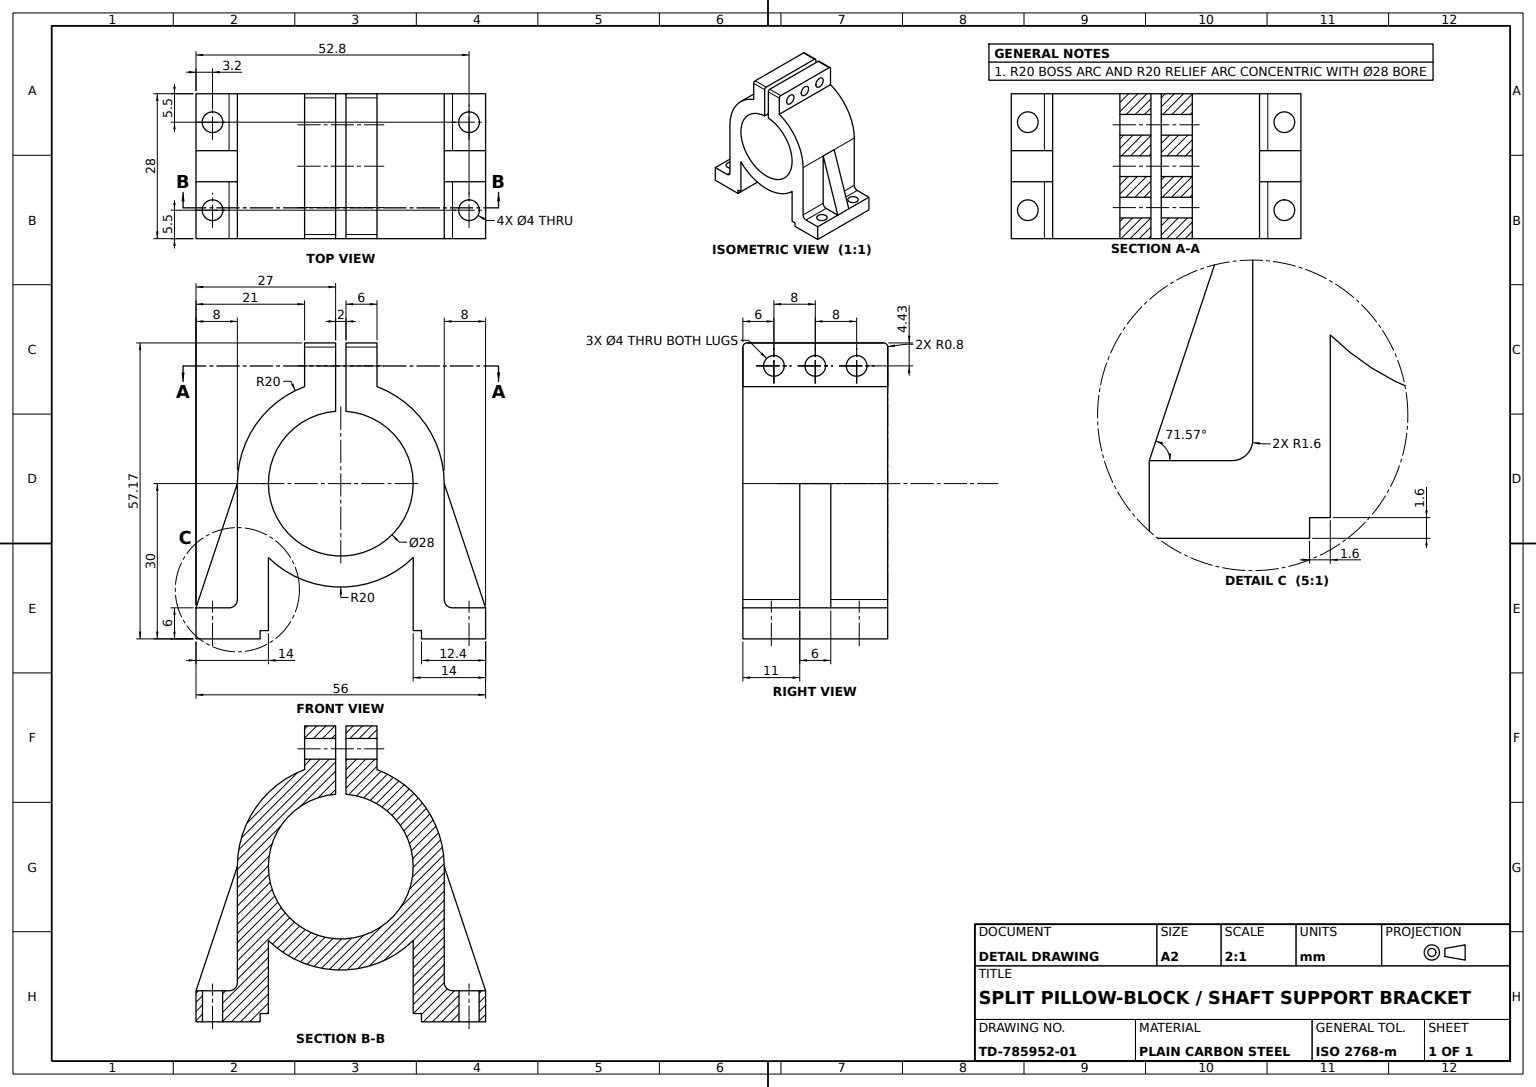
from build123d import *

# Parameters (mm, degrees)
CLAMP_BODY_DEPTH             = 28
SIDE_RECESS_A_DEPTH          = 18
SIDE_RECESS_B_DEPTH          = 18
LOWER_START                  = -28
LOWER_SIDE_BOSS_DEPTH        = 28
LOWER_BOSS_RELIEF_A_DEPTH    = 11
LOWER_START_2                = -11
LOWER_BOSS_RELIEF_B_DEPTH    = 11
UPPER_SIDE_BOSS_DEPTH        = 28
UPPER_BOSS_RELIEF_A_DEPTH    = 11
UPPER_START                  = -11
UPPER_BOSS_RELIEF_B_DEPTH    = 11
CLAMP_SCREW_HOLES_SKETCH_R   = 2
CLAMP_SCREW_HOLES_3X_DEPTH   = 20
FOOT_MOUNTING_HOLES_SKETCH_R = 2
FOOT_MOUNTING_HOLES_DEPTH    = 20


with BuildPart() as part:
    # Clamp Body Profile → Clamp Body (new body)
    with BuildSketch(Plane.XY):
        with BuildLine():
            Line((-20, 0), (-20, -22.4))
            ThreePointArc((-20, -22.4), (-20.46862915, -23.53137085), (-21.6, -24))
            Line((-21.6, -24), (-28, -24))
            Line((-28, -24), (-28, -30))
            Line((-28, -30), (-15.6, -30))
            Line((-15.6, -30), (-15.6, -28.4))
            Line((-15.6, -28.4), (-14, -28.4))
            Line((-14, -28.4), (-14, -14.282856857))
            ThreePointArc((-14, -14.282856857), (0, -20), (14, -14.282856857))
            Line((14, -14.282856857), (14, -28.4))
            Line((14, -28.4), (15.6, -28.4))
            Line((15.6, -28.4), (15.6, -30))
            Line((15.6, -30), (28, -30))
            Line((28, -30), (28, -24))
            Line((28, -24), (21.6, -24))
            ThreePointArc((21.6, -24), (20.46862915, -23.53137085), (20, -22.4))
            Line((20, -22.4), (20, 0))
            ThreePointArc((20, 0), (16.431676725, 11.401754251), (7, 18.734993995))
            Line((7, 18.734993995), (7, 27.174984355))
            Line((7, 27.174984355), (1, 27.174984355))
            Line((1, 27.174984355), (1, 19.974984355))
            Line((1, 19.974984355), (1, 13.964240044))
            ThreePointArc((1, 13.964240044), (0, -14), (-1, 13.964240044))
            Line((-1, 13.964240044), (-1, 19.974984355))
            Line((-1, 19.974984355), (-1, 27.174984355))
            Line((-1, 27.174984355), (-7, 27.174984355))
            Line((-7, 27.174984355), (-7, 18.734993995))
            ThreePointArc((-7, 18.734993995), (-16.431676725, 11.401754251), (-20, 0))
        make_face()
    extrude(amount=CLAMP_BODY_DEPTH)

    # Side Recess A Sketch → Side Recess A (cut)
    with BuildSketch(Plane(origin=(7, 0, 0), x_dir=(0, 0, -1), z_dir=(1, 0, 0))):
        with BuildLine():
            Line((-28, 26.374984355), (-28, 27.174984355))
            Line((-28, 27.174984355), (-27.2, 27.174984355))
            ThreePointArc((-27.2, 27.174984355), (-27.765685425, 26.94066978), (-28, 26.374984355))
        make_face()
    extrude(amount=-SIDE_RECESS_A_DEPTH, mode=Mode.SUBTRACT)

    # Side Recess B Sketch → Side Recess B (cut)
    with BuildSketch(Plane(origin=(7, 0, 0), x_dir=(0, 0, -1), z_dir=(1, 0, 0))):
        with BuildLine():
            Line((0, 27.174984355), (0, 26.374984355))
            ThreePointArc((0, 26.374984355), (-0.234314575, 26.94066978), (-0.8, 27.174984355))
            Line((-0.8, 27.174984355), (0, 27.174984355))
        make_face()
    extrude(amount=-SIDE_RECESS_B_DEPTH, mode=Mode.SUBTRACT)

    # Lower Side Boss Sketch → Lower Side Boss (add)
    with BuildSketch(Plane.XY.offset(28).offset(LOWER_START)):
        with BuildLine():
            Line((20, 0), (28, -24))
            Line((28, -24), (21.6, -24))
            ThreePointArc((21.6, -24), (20.46862915, -23.53137085), (20, -22.4))
            Line((20, -22.4), (20, 0))
        make_face()
    extrude(amount=LOWER_SIDE_BOSS_DEPTH)

    # Lower Boss Relief A Sketch → Lower Boss Relief A (cut)
    with BuildSketch(Plane.XY.offset(28)):
        with BuildLine():
            Line((20, 0), (28, -24))
            Line((28, -24), (21.6, -24))
            ThreePointArc((21.6, -24), (20.46862915, -23.53137085), (20, -22.4))
            Line((20, -22.4), (20, 0))
        make_face()
    extrude(amount=-LOWER_BOSS_RELIEF_A_DEPTH, mode=Mode.SUBTRACT)

    # Lower Boss Relief B Sketch → Lower Boss Relief B (cut)
    with BuildSketch(Plane(origin=(0, 0, 0), x_dir=(-1, 0, 0), z_dir=(0, 0, -1)).offset(LOWER_START_2)):
        with BuildLine():
            Line((-20, 0), (-20, -22.4))
            ThreePointArc((-20, -22.4), (-20.46862915, -23.53137085), (-21.6, -24))
            Line((-21.6, -24), (-28, -24))
            Line((-28, -24), (-20, 0))
        make_face()
    extrude(amount=LOWER_BOSS_RELIEF_B_DEPTH, mode=Mode.SUBTRACT)

    # Upper Side Boss Sketch → Upper Side Boss (add)
    with BuildSketch(Plane(origin=(0, 0, 0), x_dir=(-1, 0, 0), z_dir=(0, 0, -1))):
        with BuildLine():
            Line((20, 0), (28, -24))
            Line((28, -24), (21.6, -24))
            ThreePointArc((21.6, -24), (20.46862915, -23.53137085), (20, -22.4))
            Line((20, -22.4), (20, 0))
        make_face()
    extrude(amount=-UPPER_SIDE_BOSS_DEPTH)

    # Upper Boss Relief A Sketch → Upper Boss Relief A (cut)
    with BuildSketch(Plane(origin=(0, 0, 0), x_dir=(-1, 0, 0), z_dir=(0, 0, -1))):
        with BuildLine():
            Line((20, 0), (20, -22.4))
            ThreePointArc((20, -22.4), (20.46862915, -23.53137085), (21.6, -24))
            Line((21.6, -24), (28, -24))
            Line((28, -24), (20, 0))
        make_face()
    extrude(amount=-UPPER_BOSS_RELIEF_A_DEPTH, mode=Mode.SUBTRACT)

    # Upper Boss Relief B Sketch → Upper Boss Relief B (cut)
    with BuildSketch(Plane.XY.offset(28).offset(UPPER_START)):
        with BuildLine():
            Line((-20, 0), (-20, -22.4))
            ThreePointArc((-20, -22.4), (-20.46862915, -23.53137085), (-21.6, -24))
            Line((-21.6, -24), (-28, -24))
            Line((-28, -24), (-20, 0))
        make_face()
    extrude(amount=UPPER_BOSS_RELIEF_B_DEPTH, mode=Mode.SUBTRACT)

    # Clamp Screw Holes Sketch → Clamp Screw Holes 3x (cut)
    with BuildSketch(Plane(origin=(7, 0, 0), x_dir=(0, 0, -1), z_dir=(1, 0, 0))):
        with Locations((-22, 22.743733378)):
            Circle(CLAMP_SCREW_HOLES_SKETCH_R)
        with Locations((-14, 22.743733378)):
            Circle(CLAMP_SCREW_HOLES_SKETCH_R)
        with Locations((-6, 22.743733378)):
            Circle(CLAMP_SCREW_HOLES_SKETCH_R)
    extrude(amount=-CLAMP_SCREW_HOLES_3X_DEPTH, mode=Mode.SUBTRACT)

    # Foot Mounting Holes Sketch → Foot Mounting Holes (cut)
    with BuildSketch(Plane(origin=(0, -24, 0), x_dir=(1, 0, 0), z_dir=(0, 1, 0))):
        with Locations(Location((24.8, -22.5, 0), (0, 0, 270))):
            Circle(FOOT_MOUNTING_HOLES_SKETCH_R)
        with Locations(Location((24.8, -5.5, 0), (0, 0, 270))):
            Circle(FOOT_MOUNTING_HOLES_SKETCH_R)
        with Locations(Location((-24.8, -5.5, 0), (0, 0, 270))):
            Circle(FOOT_MOUNTING_HOLES_SKETCH_R)
        with Locations(Location((-24.8, -22.5, 0), (0, 0, 270))):
            Circle(FOOT_MOUNTING_HOLES_SKETCH_R)
    extrude(amount=-FOOT_MOUNTING_HOLES_DEPTH, mode=Mode.SUBTRACT)


solid = part.part
